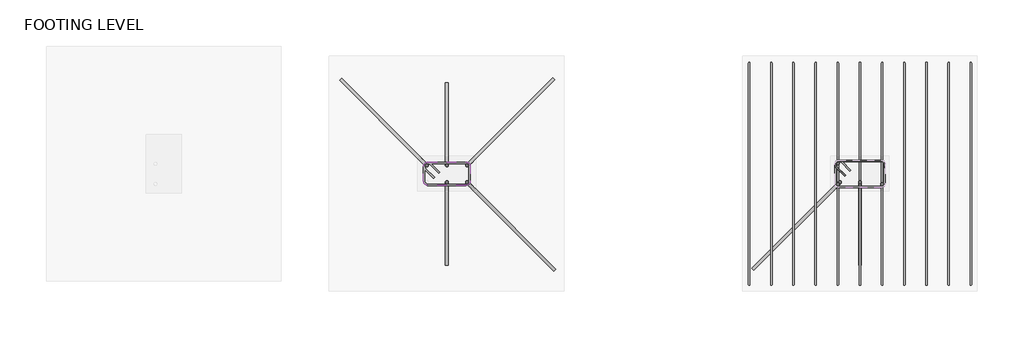
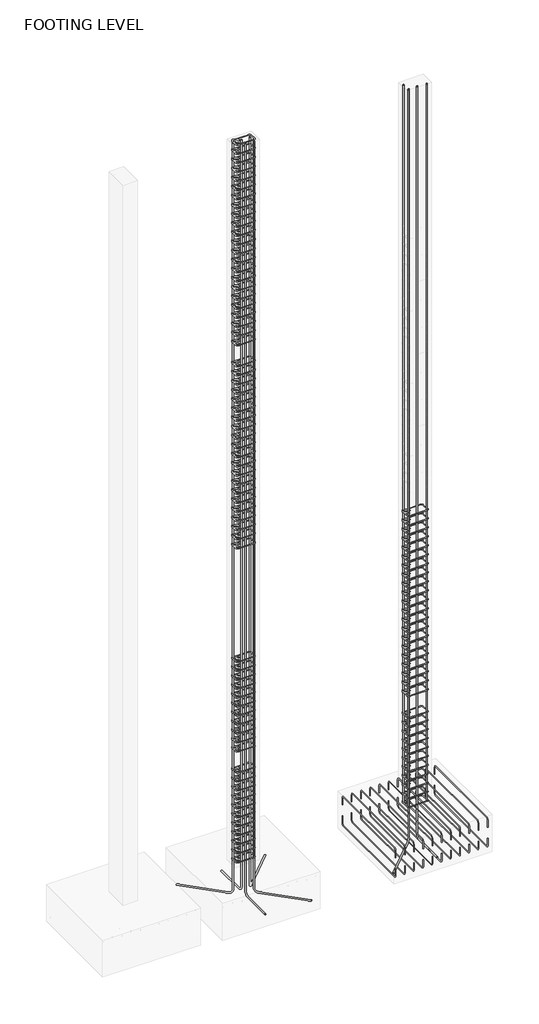
# One storey, part 4 of 10: 19 reinforcing bars.
"""IFC4 building model written with IfcOpenShell, lengths in millimetres."""

from ifc_helpers import new_model, si_unit, point, frame, origin, place, context, project, spatial, polyline, circle_curve, trimmed, segment, composite_curve, source, transform, mapped, element, save
from ifc_brep_helpers import swept_disk

model = new_model("IFC4")

# Units and contexts
model_context = context("Model", 3, world=origin())
ifc_project = project(units=[si_unit("LENGTHUNIT", "METRE", prefix="MILLI")], contexts=[model_context])

# Site, building, storey
site = spatial("IfcSite", under=ifc_project)
building = spatial("IfcBuilding", under=site)
storey = spatial("IfcBuildingStorey", under=building, Name="FOOTING LEVEL", Elevation=-1371.6)

# Reinforcing bars
placement = place(None, origin())
reinforcing_bar_shape = source(origin(), model_context, "Body", "SolidModel", [
    swept_disk(composite_curve([segment(polyline([(-10916.8793223, 5647.2626382, -1770.864029), (-10916.8793223, 5647.2626382, -1885.164029)]), True, "CONTINUOUS"), segment(trimmed(circle_curve(frame((-10916.8793223, 5613.9251382, -1885.164029), z_axis=(-1.0, 0.0, 0.0), x_axis=(0.0, 33.337499999999636, 0.0)), 33.3375), [point((-10916.8793223, 5647.2626382, -1885.164029))], [point((-10916.8793223, 5613.9251382, -1918.501529))], True, "CARTESIAN"), True, "CONTINUOUS"), segment(polyline([(-10916.8793223, 5613.9251382, -1918.501529), (-10916.8793223, 4242.3251382, -1918.501529)]), True, "CONTINUOUS"), segment(trimmed(circle_curve(frame((-10916.8793223, 4242.3251382, -1885.164029), z_axis=(-1.0, 0.0, 0.0), x_axis=(0.0, 0.0, -33.337499999999864)), 33.3375), [point((-10916.8793223, 4242.3251382, -1918.501529))], [point((-10916.8793223, 4208.9876382, -1885.164029))], True, "CARTESIAN"), True, "CONTINUOUS"), segment(polyline([(-10916.8793223, 4208.9876382, -1885.164029), (-10916.8793223, 4208.9876382, -1770.864029)]), True, "CONTINUOUS")], self_intersect=False), 4.7625),
])
element("IfcReinforcingBar", 1, at=placement, inside=storey, context=model_context, shape_type="MappedRepresentation", body=[
    mapped(reinforcing_bar_shape, transform((0.0, 0.0, 0.0), x_axis=(1.0, 0.0, 0.0), y_axis=(0.0, 1.0, 0.0), z_axis=(0.0, 0.0, 1.0))),
    mapped(reinforcing_bar_shape, transform((143.8275, 0.0, 0.0), x_axis=(1.0, 0.0, 0.0), y_axis=(0.0, 1.0, 0.0), z_axis=(0.0, 0.0, 1.0))),
    mapped(reinforcing_bar_shape, transform((287.655, 0.0, 0.0), x_axis=(1.0, 0.0, 0.0), y_axis=(0.0, 1.0, 0.0), z_axis=(0.0, 0.0, 1.0))),
    mapped(reinforcing_bar_shape, transform((431.4825, 0.0, 0.0), x_axis=(1.0, 0.0, 0.0), y_axis=(0.0, 1.0, 0.0), z_axis=(0.0, 0.0, 1.0))),
    mapped(reinforcing_bar_shape, transform((575.31, 0.0, 0.0), x_axis=(1.0, 0.0, 0.0), y_axis=(0.0, 1.0, 0.0), z_axis=(0.0, 0.0, 1.0))),
    mapped(reinforcing_bar_shape, transform((719.1375, 0.0, 0.0), x_axis=(1.0, 0.0, 0.0), y_axis=(0.0, 1.0, 0.0), z_axis=(0.0, 0.0, 1.0))),
    mapped(reinforcing_bar_shape, transform((862.965, 0.0, 0.0), x_axis=(1.0, 0.0, 0.0), y_axis=(0.0, 1.0, 0.0), z_axis=(0.0, 0.0, 1.0))),
    mapped(reinforcing_bar_shape, transform((1006.7925, 0.0, 0.0), x_axis=(1.0, 0.0, 0.0), y_axis=(0.0, 1.0, 0.0), z_axis=(0.0, 0.0, 1.0))),
    mapped(reinforcing_bar_shape, transform((1150.62, 0.0, 0.0), x_axis=(1.0, 0.0, 0.0), y_axis=(0.0, 1.0, 0.0), z_axis=(0.0, 0.0, 1.0))),
    mapped(reinforcing_bar_shape, transform((1294.4475, 0.0, 0.0), x_axis=(1.0, 0.0, 0.0), y_axis=(0.0, 1.0, 0.0), z_axis=(0.0, 0.0, 1.0))),
    mapped(reinforcing_bar_shape, transform((1438.275, 0.0, 0.0), x_axis=(1.0, 0.0, 0.0), y_axis=(0.0, 1.0, 0.0), z_axis=(0.0, 0.0, 1.0))),
])
reinforcing_bar_2_shape = source(origin(), model_context, "Body", "SolidModel", [
    swept_disk(composite_curve([segment(polyline([(-9478.6043223, 5647.2626382, -1586.5406765), (-9478.6043223, 5647.2626382, -1472.2406765)]), True, "CONTINUOUS"), segment(trimmed(circle_curve(frame((-9478.6043223, 5613.9251382, -1472.2406765), z_axis=(1.0, 0.0, 0.0), x_axis=(0.0, 33.337499999999636, 0.0)), 33.3375), [point((-9478.6043223, 5647.2626382, -1472.2406765))], [point((-9478.6043223, 5613.9251382, -1438.9031765))], True, "CARTESIAN"), True, "CONTINUOUS"), segment(polyline([(-9478.6043223, 5613.9251382, -1438.9031765), (-9478.6043223, 4242.3251382, -1438.9031765)]), True, "CONTINUOUS"), segment(trimmed(circle_curve(frame((-9478.6043223, 4242.3251382, -1472.2406765), z_axis=(1.0, 0.0, 0.0), x_axis=(0.0, 0.0, 33.33750000000009)), 33.3375), [point((-9478.6043223, 4242.3251382, -1438.9031765))], [point((-9478.6043223, 4208.9876382, -1472.2406765))], True, "CARTESIAN"), True, "CONTINUOUS"), segment(polyline([(-9478.6043223, 4208.9876382, -1472.2406765), (-9478.6043223, 4208.9876382, -1586.5406765)]), True, "CONTINUOUS")], self_intersect=False), 4.7625),
])
element("IfcReinforcingBar", 2, at=placement, inside=storey, context=model_context, shape_type="MappedRepresentation", body=[
    mapped(reinforcing_bar_2_shape, transform((0.0, 0.0, 0.0), x_axis=(1.0, 0.0, 0.0), y_axis=(0.0, 1.0, 0.0), z_axis=(0.0, 0.0, 1.0))),
    mapped(reinforcing_bar_2_shape, transform((-143.8275, 0.0, 0.0), x_axis=(1.0, 0.0, 0.0), y_axis=(0.0, 1.0, 0.0), z_axis=(0.0, 0.0, 1.0))),
    mapped(reinforcing_bar_2_shape, transform((-287.655, 0.0, 0.0), x_axis=(1.0, 0.0, 0.0), y_axis=(0.0, 1.0, 0.0), z_axis=(0.0, 0.0, 1.0))),
    mapped(reinforcing_bar_2_shape, transform((-431.4825, 0.0, 0.0), x_axis=(1.0, 0.0, 0.0), y_axis=(0.0, 1.0, 0.0), z_axis=(0.0, 0.0, 1.0))),
    mapped(reinforcing_bar_2_shape, transform((-575.31, 0.0, 0.0), x_axis=(1.0, 0.0, 0.0), y_axis=(0.0, 1.0, 0.0), z_axis=(0.0, 0.0, 1.0))),
    mapped(reinforcing_bar_2_shape, transform((-719.1375, 0.0, 0.0), x_axis=(1.0, 0.0, 0.0), y_axis=(0.0, 1.0, 0.0), z_axis=(0.0, 0.0, 1.0))),
    mapped(reinforcing_bar_2_shape, transform((-862.965, 0.0, 0.0), x_axis=(1.0, 0.0, 0.0), y_axis=(0.0, 1.0, 0.0), z_axis=(0.0, 0.0, 1.0))),
    mapped(reinforcing_bar_2_shape, transform((-1006.7925, 0.0, 0.0), x_axis=(1.0, 0.0, 0.0), y_axis=(0.0, 1.0, 0.0), z_axis=(0.0, 0.0, 1.0))),
    mapped(reinforcing_bar_2_shape, transform((-1150.62, 0.0, 0.0), x_axis=(1.0, 0.0, 0.0), y_axis=(0.0, 1.0, 0.0), z_axis=(0.0, 0.0, 1.0))),
    mapped(reinforcing_bar_2_shape, transform((-1294.4475, 0.0, 0.0), x_axis=(1.0, 0.0, 0.0), y_axis=(0.0, 1.0, 0.0), z_axis=(0.0, 0.0, 1.0))),
    mapped(reinforcing_bar_2_shape, transform((-1438.275, 0.0, 0.0), x_axis=(1.0, 0.0, 0.0), y_axis=(0.0, 1.0, 0.0), z_axis=(0.0, 0.0, 1.0))),
])
reinforcing_bar_3_shape = source(origin(), model_context, "Body", "SolidModel", [
    swept_disk(composite_curve([segment(polyline([(-10260.564645, 4948.4239213, -1337.3511872), (-10317.4288421, 5005.2881184, -1337.3511872)]), True, "CONTINUOUS"), segment(trimmed(circle_curve(frame((-10334.2668223, 4988.4501382, -1337.3511872), z_axis=(0.0, 0.0, 1.0), x_axis=(16.837980199999947, 16.837980199999947, 0.0)), 23.8125), [point((-10317.4288421, 5005.2881184, -1337.3511872))], [point((-10358.0793223, 4988.4501382, -1337.3511872))], True, "CARTESIAN"), True, "CONTINUOUS"), segment(polyline([(-10358.0793223, 4988.4501382, -1337.3511872), (-10358.0793223, 4867.8001382, -1337.3511872)]), True, "CONTINUOUS"), segment(trimmed(circle_curve(frame((-10334.2668223, 4867.8001382, -1337.3511872), z_axis=(0.0, 0.0, 1.0), x_axis=(-23.8125, 0.0, 0.0)), 23.8125), [point((-10358.0793223, 4867.8001382, -1337.3511872))], [point((-10334.2668223, 4843.9876382, -1337.3511872))], True, "CARTESIAN"), True, "CONTINUOUS"), segment(polyline([(-10334.2668223, 4843.9876382, -1337.3511872), (-10061.2168223, 4843.9876382, -1337.3511872)]), True, "CONTINUOUS"), segment(trimmed(circle_curve(frame((-10061.2168223, 4867.7620821, -1338.6969104), z_axis=(0.0, 0.056513312022656075, 0.9984018457335854), x_axis=(0.0, -23.774443899999824, 1.3457232000000658)), 23.8125), [point((-10061.2168223, 4843.9876382, -1337.3511872))], [point((-10037.4043223, 4867.7620821, -1338.6969104))], True, "CARTESIAN"), True, "CONTINUOUS"), segment(polyline([(-10037.4043223, 4867.7620821, -1338.6969104), (-10037.4043223, 4988.4881942, -1345.5304639)]), True, "CONTINUOUS"), segment(trimmed(circle_curve(frame((-10061.2168223, 4988.4881942, -1345.5304639), z_axis=(0.0, 0.056513312022656075, 0.9984018457335854), x_axis=(23.8125, 0.0, 0.0)), 23.8125), [point((-10037.4043223, 4988.4881942, -1345.5304639))], [point((-10061.2168223, 5012.2626382, -1346.8761872))], True, "CARTESIAN"), True, "CONTINUOUS"), segment(polyline([(-10061.2168223, 5012.2626382, -1346.8761872), (-10334.2668223, 5012.2626382, -1346.8761872)]), True, "CONTINUOUS"), segment(trimmed(circle_curve(frame((-10334.2668223, 4988.4501382, -1346.8761872), z_axis=(0.0, 0.0, 1.0), x_axis=(0.0, 23.8125, 0.0)), 23.8125), [point((-10334.2668223, 5012.2626382, -1346.8761872))], [point((-10351.1048026, 4971.6121579, -1346.8761872))], True, "CARTESIAN"), True, "CONTINUOUS"), segment(polyline([(-10351.1048026, 4971.6121579, -1346.8761872), (-10294.2406055, 4914.7479609, -1346.8761872)]), True, "CONTINUOUS")], self_intersect=False), 4.7625),
])
element("IfcReinforcingBar", 3, at=placement, inside=storey, context=model_context, shape_type="MappedRepresentation", body=[
    mapped(reinforcing_bar_3_shape, transform((0.0, 0.0, 0.0), x_axis=(1.0, 0.0, 0.0), y_axis=(0.0, 1.0, 0.0), z_axis=(0.0, 0.0, 1.0))),
    mapped(reinforcing_bar_3_shape, transform((0.0, 0.0, 147.1780014), x_axis=(1.0, 0.0, 0.0), y_axis=(0.0, 1.0, 0.0), z_axis=(0.0, 0.0, 1.0))),
    mapped(reinforcing_bar_3_shape, transform((0.0, 0.0, 294.3560028), x_axis=(1.0, 0.0, 0.0), y_axis=(0.0, 1.0, 0.0), z_axis=(0.0, 0.0, 1.0))),
    mapped(reinforcing_bar_3_shape, transform((0.0, 0.0, 441.5340042), x_axis=(1.0, 0.0, 0.0), y_axis=(0.0, 1.0, 0.0), z_axis=(0.0, 0.0, 1.0))),
    mapped(reinforcing_bar_3_shape, transform((0.0, 0.0, 588.7120056), x_axis=(1.0, 0.0, 0.0), y_axis=(0.0, 1.0, 0.0), z_axis=(0.0, 0.0, 1.0))),
    mapped(reinforcing_bar_3_shape, transform((0.0, 0.0, 735.890007), x_axis=(1.0, 0.0, 0.0), y_axis=(0.0, 1.0, 0.0), z_axis=(0.0, 0.0, 1.0))),
    mapped(reinforcing_bar_3_shape, transform((0.0, 0.0, 883.0680084), x_axis=(1.0, 0.0, 0.0), y_axis=(0.0, 1.0, 0.0), z_axis=(0.0, 0.0, 1.0))),
    mapped(reinforcing_bar_3_shape, transform((0.0, 0.0, 1030.2460098), x_axis=(1.0, 0.0, 0.0), y_axis=(0.0, 1.0, 0.0), z_axis=(0.0, 0.0, 1.0))),
    mapped(reinforcing_bar_3_shape, transform((0.0, 0.0, 1177.4240112), x_axis=(1.0, 0.0, 0.0), y_axis=(0.0, 1.0, 0.0), z_axis=(0.0, 0.0, 1.0))),
    mapped(reinforcing_bar_3_shape, transform((0.0, 0.0, 1324.6020126), x_axis=(1.0, 0.0, 0.0), y_axis=(0.0, 1.0, 0.0), z_axis=(0.0, 0.0, 1.0))),
    mapped(reinforcing_bar_3_shape, transform((0.0, 0.0, 1471.780014), x_axis=(1.0, 0.0, 0.0), y_axis=(0.0, 1.0, 0.0), z_axis=(0.0, 0.0, 1.0))),
])
element("IfcReinforcingBar", 4, at=placement, inside=storey, context=model_context, shape_type="SolidModel", body=[
    swept_disk(composite_curve([segment(polyline([(-10054.4816302, 4861.0649461, -1346.2), (-10054.4816302, 4861.0649461, 10490.2)]), True, "CONTINUOUS")], self_intersect=False), 9.525),
])
element("IfcReinforcingBar", 5, at=placement, inside=storey, context=model_context, shape_type="SolidModel", body=[
    swept_disk(composite_curve([segment(polyline([(-10341.0020144, 4995.1853303, -1346.2), (-10341.0020144, 4995.1853303, 10490.2)]), True, "CONTINUOUS")], self_intersect=False), 9.525),
])
element("IfcReinforcingBar", 6, at=placement, inside=storey, context=model_context, shape_type="SolidModel", body=[
    swept_disk(composite_curve([segment(polyline([(-10341.0020144, 4861.0649461, -1346.2), (-10341.0020144, 4861.0649461, 10490.2)]), True, "CONTINUOUS")], self_intersect=False), 9.525),
])
element("IfcReinforcingBar", 7, at=placement, inside=storey, context=model_context, shape_type="SolidModel", body=[
    swept_disk(composite_curve([segment(polyline([(-10892.4808347, 4309.5861258, -1910.4342608), (-10375.4483591, 4826.6186014, -1910.4342608)]), True, "CONTINUOUS"), segment(trimmed(circle_curve(frame((-10375.4483591, 4826.6186014, -1843.7592608), z_axis=(0.7071067811865229, -0.7071067811865721, 0.0), x_axis=(0.0, 0.0, -66.67499999999995)), 66.675), [point((-10375.4483591, 4826.6186014, -1910.4342608))], [point((-10328.3020144, 4873.7649461, -1843.7592608))], True, "CARTESIAN"), True, "CONTINUOUS"), segment(polyline([(-10328.3020144, 4873.7649461, -1843.7592608), (-10328.3020144, 4873.7649461, 10490.2)]), True, "CONTINUOUS")], self_intersect=False), 9.525),
])
element("IfcReinforcingBar", 8, at=placement, inside=storey, context=model_context, shape_type="SolidModel", body=[
    swept_disk(composite_curve([segment(polyline([(-10197.7418223, 4335.5350696, -1910.4342608), (-10197.7418223, 4807.0899461, -1910.4342608)]), True, "CONTINUOUS"), segment(trimmed(circle_curve(frame((-10197.7418223, 4807.0899461, -1843.7592608), z_axis=(1.0, 0.0, 0.0), x_axis=(0.0, 0.0, -66.67499999999995)), 66.675), [point((-10197.7418223, 4807.0899461, -1910.4342608))], [point((-10197.7418223, 4873.7649461, -1843.7592608))], True, "CARTESIAN"), True, "CONTINUOUS"), segment(polyline([(-10197.7418223, 4873.7649461, -1843.7592608), (-10197.7418223, 4873.7649461, 10490.2)]), True, "CONTINUOUS")], self_intersect=False), 9.525),
])
reinforcing_bar_4_shape = source(origin(), model_context, "Body", "SolidModel", [
    swept_disk(composite_curve([segment(polyline([(-12927.564645, 4935.7239213, -1328.7375), (-12984.4288421, 4992.5881184, -1328.7375)]), True, "CONTINUOUS"), segment(trimmed(circle_curve(frame((-13001.2668223, 4975.7501382, -1328.7375), z_axis=(0.0, 0.0, 1.0), x_axis=(16.837980199999947, 16.837980199999947, 0.0)), 23.8125), [point((-12984.4288421, 4992.5881184, -1328.7375))], [point((-13025.0793223, 4975.7501382, -1328.7375))], True, "CARTESIAN"), True, "CONTINUOUS"), segment(polyline([(-13025.0793223, 4975.7501382, -1328.7375), (-13025.0793223, 4880.5001382, -1328.7375)]), True, "CONTINUOUS"), segment(trimmed(circle_curve(frame((-13001.2668223, 4880.5001382, -1328.7375), z_axis=(0.0, 0.0, 1.0), x_axis=(-23.8125, 0.0, 0.0)), 23.8125), [point((-13025.0793223, 4880.5001382, -1328.7375))], [point((-13001.2668223, 4856.6876382, -1328.7375))], True, "CARTESIAN"), True, "CONTINUOUS"), segment(polyline([(-13001.2668223, 4856.6876382, -1328.7375), (-12753.6168223, 4856.6876382, -1328.7375)]), True, "CONTINUOUS"), segment(trimmed(circle_curve(frame((-12753.6168223, 4880.4473972, -1330.3214839), z_axis=(0.0, 0.06651901052377396, 0.9977851578566089), x_axis=(0.0, -23.759758999999576, 1.583983900000021)), 23.8125), [point((-12753.6168223, 4856.6876382, -1328.7375))], [point((-12729.8043223, 4880.4473972, -1330.3214839))], True, "CARTESIAN"), True, "CONTINUOUS"), segment(polyline([(-12729.8043223, 4880.4473972, -1330.3214839), (-12729.8043223, 4975.8028791, -1336.6785161)]), True, "CONTINUOUS"), segment(trimmed(circle_curve(frame((-12753.6168223, 4975.8028791, -1336.6785161), z_axis=(0.0, 0.06651901052377396, 0.9977851578566089), x_axis=(23.8125, 0.0, 0.0)), 23.8125), [point((-12729.8043223, 4975.8028791, -1336.6785161))], [point((-12753.6168223, 4999.5626382, -1338.2625))], True, "CARTESIAN"), True, "CONTINUOUS"), segment(polyline([(-12753.6168223, 4999.5626382, -1338.2625), (-13001.2668223, 4999.5626382, -1338.2625)]), True, "CONTINUOUS"), segment(trimmed(circle_curve(frame((-13001.2668223, 4975.7501382, -1338.2625), z_axis=(0.0, 0.0, 1.0), x_axis=(0.0, 23.8125, 0.0)), 23.8125), [point((-13001.2668223, 4999.5626382, -1338.2625))], [point((-13018.1048026, 4958.9121579, -1338.2625))], True, "CARTESIAN"), True, "CONTINUOUS"), segment(polyline([(-13018.1048026, 4958.9121579, -1338.2625), (-12961.2406055, 4902.0479609, -1338.2625)]), True, "CONTINUOUS")], self_intersect=False), 4.7625),
])
element("IfcReinforcingBar", 9, at=placement, inside=storey, context=model_context, shape_type="MappedRepresentation", body=[
    mapped(reinforcing_bar_4_shape, transform((0.0, 0.0, 0.0), x_axis=(1.0, 0.0, 0.0), y_axis=(0.0, 1.0, 0.0), z_axis=(0.0, 0.0, 1.0))),
    mapped(reinforcing_bar_4_shape, transform((0.0, 0.0, 148.11375), x_axis=(1.0, 0.0, 0.0), y_axis=(0.0, 1.0, 0.0), z_axis=(0.0, 0.0, 1.0))),
    mapped(reinforcing_bar_4_shape, transform((0.0, 0.0, 296.2275), x_axis=(1.0, 0.0, 0.0), y_axis=(0.0, 1.0, 0.0), z_axis=(0.0, 0.0, 1.0))),
    mapped(reinforcing_bar_4_shape, transform((0.0, 0.0, 444.34125), x_axis=(1.0, 0.0, 0.0), y_axis=(0.0, 1.0, 0.0), z_axis=(0.0, 0.0, 1.0))),
    mapped(reinforcing_bar_4_shape, transform((0.0, 0.0, 592.455), x_axis=(1.0, 0.0, 0.0), y_axis=(0.0, 1.0, 0.0), z_axis=(0.0, 0.0, 1.0))),
    mapped(reinforcing_bar_4_shape, transform((0.0, 0.0, 740.56875), x_axis=(1.0, 0.0, 0.0), y_axis=(0.0, 1.0, 0.0), z_axis=(0.0, 0.0, 1.0))),
    mapped(reinforcing_bar_4_shape, transform((0.0, 0.0, 888.6825), x_axis=(1.0, 0.0, 0.0), y_axis=(0.0, 1.0, 0.0), z_axis=(0.0, 0.0, 1.0))),
    mapped(reinforcing_bar_4_shape, transform((0.0, 0.0, 1036.79625), x_axis=(1.0, 0.0, 0.0), y_axis=(0.0, 1.0, 0.0), z_axis=(0.0, 0.0, 1.0))),
    mapped(reinforcing_bar_4_shape, transform((0.0, 0.0, 1184.91), x_axis=(1.0, 0.0, 0.0), y_axis=(0.0, 1.0, 0.0), z_axis=(0.0, 0.0, 1.0))),
    mapped(reinforcing_bar_4_shape, transform((0.0, 0.0, 1333.02375), x_axis=(1.0, 0.0, 0.0), y_axis=(0.0, 1.0, 0.0), z_axis=(0.0, 0.0, 1.0))),
    mapped(reinforcing_bar_4_shape, transform((0.0, 0.0, 1481.1375), x_axis=(1.0, 0.0, 0.0), y_axis=(0.0, 1.0, 0.0), z_axis=(0.0, 0.0, 1.0))),
])
element("IfcReinforcingBar", 10, at=placement, inside=storey, context=model_context, shape_type="SolidModel", body=[
    swept_disk(composite_curve([segment(polyline([(-12746.8816302, 4873.7649461, -1333.5), (-12746.8816302, 4873.7649461, 10477.5)]), True, "CONTINUOUS")], self_intersect=False), 9.525),
])
element("IfcReinforcingBar", 11, at=placement, inside=storey, context=model_context, shape_type="SolidModel", body=[
    swept_disk(composite_curve([segment(polyline([(-12185.2058743, 5544.1610861, -1910.4342608), (-12699.7352856, 5029.6316749, -1910.4342608)]), True, "CONTINUOUS"), segment(trimmed(circle_curve(frame((-12699.7352856, 5029.6316749, -1843.7592608), z_axis=(-0.7071067811865185, 0.7071067811865767, 0.0), x_axis=(0.0, 0.0, -66.67499999999995)), 66.675), [point((-12699.7352856, 5029.6316749, -1910.4342608))], [point((-12746.8816302, 4982.4853303, -1843.7592608))], True, "CARTESIAN"), True, "CONTINUOUS"), segment(polyline([(-12746.8816302, 4982.4853303, -1843.7592608), (-12746.8816302, 4982.4853303, 10477.5)]), True, "CONTINUOUS")], self_intersect=False), 9.525),
])
element("IfcReinforcingBar", 12, at=placement, inside=storey, context=model_context, shape_type="SolidModel", body=[
    swept_disk(composite_curve([segment(polyline([(-12177.1874965, 4304.0708123, -1910.4342608), (-12699.7352856, 4826.6186014, -1910.4342608)]), True, "CONTINUOUS"), segment(trimmed(circle_curve(frame((-12699.7352856, 4826.6186014, -1843.7592608), z_axis=(0.7071067811865269, 0.7071067811865681, 0.0), x_axis=(0.0, 0.0, -66.67499999999995)), 66.675), [point((-12699.7352856, 4826.6186014, -1910.4342608))], [point((-12746.8816302, 4873.7649461, -1843.7592608))], True, "CARTESIAN"), True, "CONTINUOUS"), segment(polyline([(-12746.8816302, 4873.7649461, -1843.7592608), (-12746.8816302, 4873.7649461, 10477.5)]), True, "CONTINUOUS")], self_intersect=False), 9.525),
])
element("IfcReinforcingBar", 13, at=placement, inside=storey, context=model_context, shape_type="SolidModel", body=[
    swept_disk(composite_curve([segment(polyline([(-13566.7211349, 5541.2044507, -1910.4342608), (-13055.1483591, 5029.6316749, -1910.4342608)]), True, "CONTINUOUS"), segment(trimmed(circle_curve(frame((-13055.1483591, 5029.6316749, -1843.7592608), z_axis=(-0.7071067811865223, -0.7071067811865729, 0.0), x_axis=(0.0, 0.0, -66.67499999999995)), 66.675), [point((-13055.1483591, 5029.6316749, -1910.4342608))], [point((-13008.0020144, 4982.4853303, -1843.7592608))], True, "CARTESIAN"), True, "CONTINUOUS"), segment(polyline([(-13008.0020144, 4982.4853303, -1843.7592608), (-13008.0020144, 4982.4853303, 10477.5)]), True, "CONTINUOUS")], self_intersect=False), 9.525),
])
element("IfcReinforcingBar", 14, at=placement, inside=storey, context=model_context, shape_type="SolidModel", body=[
    swept_disk(composite_curve([segment(polyline([(-12877.4418223, 5520.7152067, -1910.4342608), (-12877.4418223, 5049.1603303, -1910.4342608)]), True, "CONTINUOUS"), segment(trimmed(circle_curve(frame((-12877.4418223, 5049.1603303, -1843.7592608), z_axis=(-1.0, 0.0, 0.0), x_axis=(0.0, 0.0, -66.67499999999995)), 66.675), [point((-12877.4418223, 5049.1603303, -1910.4342608))], [point((-12877.4418223, 4982.4853303, -1843.7592608))], True, "CARTESIAN"), True, "CONTINUOUS"), segment(polyline([(-12877.4418223, 4982.4853303, -1843.7592608), (-12877.4418223, 4982.4853303, 10477.5)]), True, "CONTINUOUS")], self_intersect=False), 9.525),
])
element("IfcReinforcingBar", 15, at=placement, inside=storey, context=model_context, shape_type="SolidModel", body=[
    swept_disk(composite_curve([segment(polyline([(-12877.4418223, 4335.5350696, -1910.4342608), (-12877.4418223, 4807.0899461, -1910.4342608)]), True, "CONTINUOUS"), segment(trimmed(circle_curve(frame((-12877.4418223, 4807.0899461, -1843.7592608), z_axis=(1.0, 0.0, 0.0), x_axis=(0.0, 0.0, -66.67499999999995)), 66.675), [point((-12877.4418223, 4807.0899461, -1910.4342608))], [point((-12877.4418223, 4873.7649461, -1843.7592608))], True, "CARTESIAN"), True, "CONTINUOUS"), segment(polyline([(-12877.4418223, 4873.7649461, -1843.7592608), (-12877.4418223, 4873.7649461, 10477.5)]), True, "CONTINUOUS")], self_intersect=False), 9.525),
])
reinforcing_bar_5_shape = source(origin(), model_context, "Body", "SolidModel", [
    swept_disk(composite_curve([segment(polyline([(-10260.564645, 4948.4239213, 491.4488128), (-10317.4288421, 5005.2881184, 491.4488128)]), True, "CONTINUOUS"), segment(trimmed(circle_curve(frame((-10334.2668223, 4988.4501382, 491.4488128), z_axis=(0.0, 0.0, 1.0), x_axis=(16.837980199999947, 16.837980199999947, 0.0)), 23.8125), [point((-10317.4288421, 5005.2881184, 491.4488128))], [point((-10358.0793223, 4988.4501382, 491.4488128))], True, "CARTESIAN"), True, "CONTINUOUS"), segment(polyline([(-10358.0793223, 4988.4501382, 491.4488128), (-10358.0793223, 4867.8001382, 491.4488128)]), True, "CONTINUOUS"), segment(trimmed(circle_curve(frame((-10334.2668223, 4867.8001382, 491.4488128), z_axis=(0.0, 0.0, 1.0), x_axis=(-23.8125, 0.0, 0.0)), 23.8125), [point((-10358.0793223, 4867.8001382, 491.4488128))], [point((-10334.2668223, 4843.9876382, 491.4488128))], True, "CARTESIAN"), True, "CONTINUOUS"), segment(polyline([(-10334.2668223, 4843.9876382, 491.4488128), (-10061.2168223, 4843.9876382, 491.4488128)]), True, "CONTINUOUS"), segment(trimmed(circle_curve(frame((-10061.2168223, 4867.7620821, 490.1030896), z_axis=(0.0, 0.056513312022656075, 0.9984018457335854), x_axis=(0.0, -23.774443899999824, 1.345723200000009)), 23.8125), [point((-10061.2168223, 4843.9876382, 491.4488128))], [point((-10037.4043223, 4867.7620821, 490.1030896))], True, "CARTESIAN"), True, "CONTINUOUS"), segment(polyline([(-10037.4043223, 4867.7620821, 490.1030896), (-10037.4043223, 4988.4881942, 483.2695361)]), True, "CONTINUOUS"), segment(trimmed(circle_curve(frame((-10061.2168223, 4988.4881942, 483.2695361), z_axis=(0.0, 0.056513312022656075, 0.9984018457335854), x_axis=(23.8125, 0.0, 0.0)), 23.8125), [point((-10037.4043223, 4988.4881942, 483.2695361))], [point((-10061.2168223, 5012.2626382, 481.9238128))], True, "CARTESIAN"), True, "CONTINUOUS"), segment(polyline([(-10061.2168223, 5012.2626382, 481.9238128), (-10334.2668223, 5012.2626382, 481.9238128)]), True, "CONTINUOUS"), segment(trimmed(circle_curve(frame((-10334.2668223, 4988.4501382, 481.9238128), z_axis=(0.0, 0.0, 1.0), x_axis=(0.0, 23.8125, 0.0)), 23.8125), [point((-10334.2668223, 5012.2626382, 481.9238128))], [point((-10351.1048026, 4971.6121579, 481.9238128))], True, "CARTESIAN"), True, "CONTINUOUS"), segment(polyline([(-10351.1048026, 4971.6121579, 481.9238128), (-10294.2406055, 4914.7479609, 481.9238128)]), True, "CONTINUOUS")], self_intersect=False), 4.7625),
])
element("IfcReinforcingBar", 16, at=placement, inside=storey, context=model_context, shape_type="MappedRepresentation", body=[
    mapped(reinforcing_bar_5_shape, transform((0.0, 0.0, 0.0), x_axis=(1.0, 0.0, 0.0), y_axis=(0.0, 1.0, 0.0), z_axis=(0.0, 0.0, 1.0))),
    mapped(reinforcing_bar_5_shape, transform((0.0, 0.0, 148.5671059), x_axis=(1.0, 0.0, 0.0), y_axis=(0.0, 1.0, 0.0), z_axis=(0.0, 0.0, 1.0))),
    mapped(reinforcing_bar_5_shape, transform((0.0, 0.0, 297.1342118), x_axis=(1.0, 0.0, 0.0), y_axis=(0.0, 1.0, 0.0), z_axis=(0.0, 0.0, 1.0))),
    mapped(reinforcing_bar_5_shape, transform((0.0, 0.0, 445.7013177), x_axis=(1.0, 0.0, 0.0), y_axis=(0.0, 1.0, 0.0), z_axis=(0.0, 0.0, 1.0))),
    mapped(reinforcing_bar_5_shape, transform((0.0, 0.0, 594.2684236), x_axis=(1.0, 0.0, 0.0), y_axis=(0.0, 1.0, 0.0), z_axis=(0.0, 0.0, 1.0))),
    mapped(reinforcing_bar_5_shape, transform((0.0, 0.0, 742.8355295), x_axis=(1.0, 0.0, 0.0), y_axis=(0.0, 1.0, 0.0), z_axis=(0.0, 0.0, 1.0))),
    mapped(reinforcing_bar_5_shape, transform((0.0, 0.0, 891.4026354), x_axis=(1.0, 0.0, 0.0), y_axis=(0.0, 1.0, 0.0), z_axis=(0.0, 0.0, 1.0))),
    mapped(reinforcing_bar_5_shape, transform((0.0, 0.0, 1039.9697413), x_axis=(1.0, 0.0, 0.0), y_axis=(0.0, 1.0, 0.0), z_axis=(0.0, 0.0, 1.0))),
    mapped(reinforcing_bar_5_shape, transform((0.0, 0.0, 1188.5368472), x_axis=(1.0, 0.0, 0.0), y_axis=(0.0, 1.0, 0.0), z_axis=(0.0, 0.0, 1.0))),
    mapped(reinforcing_bar_5_shape, transform((0.0, 0.0, 1337.1039531), x_axis=(1.0, 0.0, 0.0), y_axis=(0.0, 1.0, 0.0), z_axis=(0.0, 0.0, 1.0))),
    mapped(reinforcing_bar_5_shape, transform((0.0, 0.0, 1485.671059), x_axis=(1.0, 0.0, 0.0), y_axis=(0.0, 1.0, 0.0), z_axis=(0.0, 0.0, 1.0))),
    mapped(reinforcing_bar_5_shape, transform((0.0, 0.0, 1634.2381649), x_axis=(1.0, 0.0, 0.0), y_axis=(0.0, 1.0, 0.0), z_axis=(0.0, 0.0, 1.0))),
    mapped(reinforcing_bar_5_shape, transform((0.0, 0.0, 1782.8052708), x_axis=(1.0, 0.0, 0.0), y_axis=(0.0, 1.0, 0.0), z_axis=(0.0, 0.0, 1.0))),
    mapped(reinforcing_bar_5_shape, transform((0.0, 0.0, 1931.3723767), x_axis=(1.0, 0.0, 0.0), y_axis=(0.0, 1.0, 0.0), z_axis=(0.0, 0.0, 1.0))),
    mapped(reinforcing_bar_5_shape, transform((0.0, 0.0, 2079.9394826), x_axis=(1.0, 0.0, 0.0), y_axis=(0.0, 1.0, 0.0), z_axis=(0.0, 0.0, 1.0))),
    mapped(reinforcing_bar_5_shape, transform((0.0, 0.0, 2228.5065885), x_axis=(1.0, 0.0, 0.0), y_axis=(0.0, 1.0, 0.0), z_axis=(0.0, 0.0, 1.0))),
    mapped(reinforcing_bar_5_shape, transform((0.0, 0.0, 2377.0736944), x_axis=(1.0, 0.0, 0.0), y_axis=(0.0, 1.0, 0.0), z_axis=(0.0, 0.0, 1.0))),
    mapped(reinforcing_bar_5_shape, transform((0.0, 0.0, 2525.6408003), x_axis=(1.0, 0.0, 0.0), y_axis=(0.0, 1.0, 0.0), z_axis=(0.0, 0.0, 1.0))),
    mapped(reinforcing_bar_5_shape, transform((0.0, 0.0, 2674.2079062), x_axis=(1.0, 0.0, 0.0), y_axis=(0.0, 1.0, 0.0), z_axis=(0.0, 0.0, 1.0))),
    mapped(reinforcing_bar_5_shape, transform((0.0, 0.0, 2822.775012), x_axis=(1.0, 0.0, 0.0), y_axis=(0.0, 1.0, 0.0), z_axis=(0.0, 0.0, 1.0))),
    mapped(reinforcing_bar_5_shape, transform((0.0, 0.0, 2971.3421179), x_axis=(1.0, 0.0, 0.0), y_axis=(0.0, 1.0, 0.0), z_axis=(0.0, 0.0, 1.0))),
])
reinforcing_bar_6_shape = source(origin(), model_context, "Body", "SolidModel", [
    swept_disk(composite_curve([segment(polyline([(-12927.564645, 4935.7239213, 500.0625), (-12984.4288421, 4992.5881184, 500.0625)]), True, "CONTINUOUS"), segment(trimmed(circle_curve(frame((-13001.2668223, 4975.7501382, 500.0625), z_axis=(0.0, 0.0, 1.0), x_axis=(16.837980199999947, 16.837980199999947, 0.0)), 23.8125), [point((-12984.4288421, 4992.5881184, 500.0625))], [point((-13025.0793223, 4975.7501382, 500.0625))], True, "CARTESIAN"), True, "CONTINUOUS"), segment(polyline([(-13025.0793223, 4975.7501382, 500.0625), (-13025.0793223, 4880.5001382, 500.0625)]), True, "CONTINUOUS"), segment(trimmed(circle_curve(frame((-13001.2668223, 4880.5001382, 500.0625), z_axis=(0.0, 0.0, 1.0), x_axis=(-23.8125, 0.0, 0.0)), 23.8125), [point((-13025.0793223, 4880.5001382, 500.0625))], [point((-13001.2668223, 4856.6876382, 500.0625))], True, "CARTESIAN"), True, "CONTINUOUS"), segment(polyline([(-13001.2668223, 4856.6876382, 500.0625), (-12753.6168223, 4856.6876382, 500.0625)]), True, "CONTINUOUS"), segment(trimmed(circle_curve(frame((-12753.6168223, 4880.4473972, 498.4785161), z_axis=(0.0, 0.06651901052377396, 0.9977851578566089), x_axis=(0.0, -23.759758999999576, 1.583983900000021)), 23.8125), [point((-12753.6168223, 4856.6876382, 500.0625))], [point((-12729.8043223, 4880.4473972, 498.4785161))], True, "CARTESIAN"), True, "CONTINUOUS"), segment(polyline([(-12729.8043223, 4880.4473972, 498.4785161), (-12729.8043223, 4975.8028791, 492.1214839)]), True, "CONTINUOUS"), segment(trimmed(circle_curve(frame((-12753.6168223, 4975.8028791, 492.1214839), z_axis=(0.0, 0.06651901052377396, 0.9977851578566089), x_axis=(23.8125, 0.0, 0.0)), 23.8125), [point((-12729.8043223, 4975.8028791, 492.1214839))], [point((-12753.6168223, 4999.5626382, 490.5375))], True, "CARTESIAN"), True, "CONTINUOUS"), segment(polyline([(-12753.6168223, 4999.5626382, 490.5375), (-13001.2668223, 4999.5626382, 490.5375)]), True, "CONTINUOUS"), segment(trimmed(circle_curve(frame((-13001.2668223, 4975.7501382, 490.5375), z_axis=(0.0, 0.0, 1.0), x_axis=(0.0, 23.8125, 0.0)), 23.8125), [point((-13001.2668223, 4999.5626382, 490.5375))], [point((-13018.1048026, 4958.9121579, 490.5375))], True, "CARTESIAN"), True, "CONTINUOUS"), segment(polyline([(-13018.1048026, 4958.9121579, 490.5375), (-12961.2406055, 4902.0479609, 490.5375)]), True, "CONTINUOUS")], self_intersect=False), 4.7625),
])
element("IfcReinforcingBar", 17, at=placement, inside=storey, context=model_context, shape_type="MappedRepresentation", body=[
    mapped(reinforcing_bar_6_shape, transform((0.0, 0.0, 0.0), x_axis=(1.0, 0.0, 0.0), y_axis=(0.0, 1.0, 0.0), z_axis=(0.0, 0.0, 1.0))),
    mapped(reinforcing_bar_6_shape, transform((0.0, 0.0, 148.11375), x_axis=(1.0, 0.0, 0.0), y_axis=(0.0, 1.0, 0.0), z_axis=(0.0, 0.0, 1.0))),
    mapped(reinforcing_bar_6_shape, transform((0.0, 0.0, 296.2275), x_axis=(1.0, 0.0, 0.0), y_axis=(0.0, 1.0, 0.0), z_axis=(0.0, 0.0, 1.0))),
    mapped(reinforcing_bar_6_shape, transform((0.0, 0.0, 444.34125), x_axis=(1.0, 0.0, 0.0), y_axis=(0.0, 1.0, 0.0), z_axis=(0.0, 0.0, 1.0))),
    mapped(reinforcing_bar_6_shape, transform((0.0, 0.0, 592.455), x_axis=(1.0, 0.0, 0.0), y_axis=(0.0, 1.0, 0.0), z_axis=(0.0, 0.0, 1.0))),
    mapped(reinforcing_bar_6_shape, transform((0.0, 0.0, 740.56875), x_axis=(1.0, 0.0, 0.0), y_axis=(0.0, 1.0, 0.0), z_axis=(0.0, 0.0, 1.0))),
    mapped(reinforcing_bar_6_shape, transform((0.0, 0.0, 888.6825), x_axis=(1.0, 0.0, 0.0), y_axis=(0.0, 1.0, 0.0), z_axis=(0.0, 0.0, 1.0))),
    mapped(reinforcing_bar_6_shape, transform((0.0, 0.0, 1036.79625), x_axis=(1.0, 0.0, 0.0), y_axis=(0.0, 1.0, 0.0), z_axis=(0.0, 0.0, 1.0))),
    mapped(reinforcing_bar_6_shape, transform((0.0, 0.0, 1184.91), x_axis=(1.0, 0.0, 0.0), y_axis=(0.0, 1.0, 0.0), z_axis=(0.0, 0.0, 1.0))),
    mapped(reinforcing_bar_6_shape, transform((0.0, 0.0, 1333.02375), x_axis=(1.0, 0.0, 0.0), y_axis=(0.0, 1.0, 0.0), z_axis=(0.0, 0.0, 1.0))),
    mapped(reinforcing_bar_6_shape, transform((0.0, 0.0, 1481.1375), x_axis=(1.0, 0.0, 0.0), y_axis=(0.0, 1.0, 0.0), z_axis=(0.0, 0.0, 1.0))),
])
reinforcing_bar_7_shape = source(origin(), model_context, "Body", "SolidModel", [
    swept_disk(composite_curve([segment(polyline([(-12927.564645, 4935.7239213, 3852.8625), (-12984.4288421, 4992.5881184, 3852.8625)]), True, "CONTINUOUS"), segment(trimmed(circle_curve(frame((-13001.2668223, 4975.7501382, 3852.8625), z_axis=(0.0, 0.0, 1.0), x_axis=(16.837980199999947, 16.837980199999947, 0.0)), 23.8125), [point((-12984.4288421, 4992.5881184, 3852.8625))], [point((-13025.0793223, 4975.7501382, 3852.8625))], True, "CARTESIAN"), True, "CONTINUOUS"), segment(polyline([(-13025.0793223, 4975.7501382, 3852.8625), (-13025.0793223, 4880.5001382, 3852.8625)]), True, "CONTINUOUS"), segment(trimmed(circle_curve(frame((-13001.2668223, 4880.5001382, 3852.8625), z_axis=(0.0, 0.0, 1.0), x_axis=(-23.8125, 0.0, 0.0)), 23.8125), [point((-13025.0793223, 4880.5001382, 3852.8625))], [point((-13001.2668223, 4856.6876382, 3852.8625))], True, "CARTESIAN"), True, "CONTINUOUS"), segment(polyline([(-13001.2668223, 4856.6876382, 3852.8625), (-12753.6168223, 4856.6876382, 3852.8625)]), True, "CONTINUOUS"), segment(trimmed(circle_curve(frame((-12753.6168223, 4880.4473972, 3851.2785161), z_axis=(0.0, 0.06651901052377396, 0.9977851578566089), x_axis=(0.0, -23.759758999999576, 1.583983900000021)), 23.8125), [point((-12753.6168223, 4856.6876382, 3852.8625))], [point((-12729.8043223, 4880.4473972, 3851.2785161))], True, "CARTESIAN"), True, "CONTINUOUS"), segment(polyline([(-12729.8043223, 4880.4473972, 3851.2785161), (-12729.8043223, 4975.8028791, 3844.9214839)]), True, "CONTINUOUS"), segment(trimmed(circle_curve(frame((-12753.6168223, 4975.8028791, 3844.9214839), z_axis=(0.0, 0.06651901052377396, 0.9977851578566089), x_axis=(23.8125, 0.0, 0.0)), 23.8125), [point((-12729.8043223, 4975.8028791, 3844.9214839))], [point((-12753.6168223, 4999.5626382, 3843.3375))], True, "CARTESIAN"), True, "CONTINUOUS"), segment(polyline([(-12753.6168223, 4999.5626382, 3843.3375), (-13001.2668223, 4999.5626382, 3843.3375)]), True, "CONTINUOUS"), segment(trimmed(circle_curve(frame((-13001.2668223, 4975.7501382, 3843.3375), z_axis=(0.0, 0.0, 1.0), x_axis=(0.0, 23.8125, 0.0)), 23.8125), [point((-13001.2668223, 4999.5626382, 3843.3375))], [point((-13018.1048026, 4958.9121579, 3843.3375))], True, "CARTESIAN"), True, "CONTINUOUS"), segment(polyline([(-13018.1048026, 4958.9121579, 3843.3375), (-12961.2406055, 4902.0479609, 3843.3375)]), True, "CONTINUOUS")], self_intersect=False), 4.7625),
])
element("IfcReinforcingBar", 18, at=placement, inside=storey, context=model_context, shape_type="MappedRepresentation", body=[
    mapped(reinforcing_bar_7_shape, transform((0.0, 0.0, 0.0), x_axis=(1.0, 0.0, 0.0), y_axis=(0.0, 1.0, 0.0), z_axis=(0.0, 0.0, 1.0))),
    mapped(reinforcing_bar_7_shape, transform((0.0, 0.0, 150.256875), x_axis=(1.0, 0.0, 0.0), y_axis=(0.0, 1.0, 0.0), z_axis=(0.0, 0.0, 1.0))),
    mapped(reinforcing_bar_7_shape, transform((0.0, 0.0, 300.51375), x_axis=(1.0, 0.0, 0.0), y_axis=(0.0, 1.0, 0.0), z_axis=(0.0, 0.0, 1.0))),
    mapped(reinforcing_bar_7_shape, transform((0.0, 0.0, 450.770625), x_axis=(1.0, 0.0, 0.0), y_axis=(0.0, 1.0, 0.0), z_axis=(0.0, 0.0, 1.0))),
    mapped(reinforcing_bar_7_shape, transform((0.0, 0.0, 601.0275), x_axis=(1.0, 0.0, 0.0), y_axis=(0.0, 1.0, 0.0), z_axis=(0.0, 0.0, 1.0))),
    mapped(reinforcing_bar_7_shape, transform((0.0, 0.0, 751.284375), x_axis=(1.0, 0.0, 0.0), y_axis=(0.0, 1.0, 0.0), z_axis=(0.0, 0.0, 1.0))),
    mapped(reinforcing_bar_7_shape, transform((0.0, 0.0, 901.54125), x_axis=(1.0, 0.0, 0.0), y_axis=(0.0, 1.0, 0.0), z_axis=(0.0, 0.0, 1.0))),
    mapped(reinforcing_bar_7_shape, transform((0.0, 0.0, 1051.798125), x_axis=(1.0, 0.0, 0.0), y_axis=(0.0, 1.0, 0.0), z_axis=(0.0, 0.0, 1.0))),
    mapped(reinforcing_bar_7_shape, transform((0.0, 0.0, 1202.055), x_axis=(1.0, 0.0, 0.0), y_axis=(0.0, 1.0, 0.0), z_axis=(0.0, 0.0, 1.0))),
    mapped(reinforcing_bar_7_shape, transform((0.0, 0.0, 1352.311875), x_axis=(1.0, 0.0, 0.0), y_axis=(0.0, 1.0, 0.0), z_axis=(0.0, 0.0, 1.0))),
    mapped(reinforcing_bar_7_shape, transform((0.0, 0.0, 1502.56875), x_axis=(1.0, 0.0, 0.0), y_axis=(0.0, 1.0, 0.0), z_axis=(0.0, 0.0, 1.0))),
    mapped(reinforcing_bar_7_shape, transform((0.0, 0.0, 1652.825625), x_axis=(1.0, 0.0, 0.0), y_axis=(0.0, 1.0, 0.0), z_axis=(0.0, 0.0, 1.0))),
    mapped(reinforcing_bar_7_shape, transform((0.0, 0.0, 1803.0825), x_axis=(1.0, 0.0, 0.0), y_axis=(0.0, 1.0, 0.0), z_axis=(0.0, 0.0, 1.0))),
    mapped(reinforcing_bar_7_shape, transform((0.0, 0.0, 1953.339375), x_axis=(1.0, 0.0, 0.0), y_axis=(0.0, 1.0, 0.0), z_axis=(0.0, 0.0, 1.0))),
    mapped(reinforcing_bar_7_shape, transform((0.0, 0.0, 2103.59625), x_axis=(1.0, 0.0, 0.0), y_axis=(0.0, 1.0, 0.0), z_axis=(0.0, 0.0, 1.0))),
    mapped(reinforcing_bar_7_shape, transform((0.0, 0.0, 2253.853125), x_axis=(1.0, 0.0, 0.0), y_axis=(0.0, 1.0, 0.0), z_axis=(0.0, 0.0, 1.0))),
    mapped(reinforcing_bar_7_shape, transform((0.0, 0.0, 2404.11), x_axis=(1.0, 0.0, 0.0), y_axis=(0.0, 1.0, 0.0), z_axis=(0.0, 0.0, 1.0))),
    mapped(reinforcing_bar_7_shape, transform((0.0, 0.0, 2554.366875), x_axis=(1.0, 0.0, 0.0), y_axis=(0.0, 1.0, 0.0), z_axis=(0.0, 0.0, 1.0))),
    mapped(reinforcing_bar_7_shape, transform((0.0, 0.0, 2704.62375), x_axis=(1.0, 0.0, 0.0), y_axis=(0.0, 1.0, 0.0), z_axis=(0.0, 0.0, 1.0))),
    mapped(reinforcing_bar_7_shape, transform((0.0, 0.0, 2854.880625), x_axis=(1.0, 0.0, 0.0), y_axis=(0.0, 1.0, 0.0), z_axis=(0.0, 0.0, 1.0))),
    mapped(reinforcing_bar_7_shape, transform((0.0, 0.0, 3005.1375), x_axis=(1.0, 0.0, 0.0), y_axis=(0.0, 1.0, 0.0), z_axis=(0.0, 0.0, 1.0))),
])
reinforcing_bar_8_shape = source(origin(), model_context, "Body", "SolidModel", [
    swept_disk(composite_curve([segment(polyline([(-12927.564645, 4935.7239213, 7205.6625), (-12984.4288421, 4992.5881184, 7205.6625)]), True, "CONTINUOUS"), segment(trimmed(circle_curve(frame((-13001.2668223, 4975.7501382, 7205.6625), z_axis=(0.0, 0.0, 1.0), x_axis=(16.837980199999947, 16.837980199999947, 0.0)), 23.8125), [point((-12984.4288421, 4992.5881184, 7205.6625))], [point((-13025.0793223, 4975.7501382, 7205.6625))], True, "CARTESIAN"), True, "CONTINUOUS"), segment(polyline([(-13025.0793223, 4975.7501382, 7205.6625), (-13025.0793223, 4880.5001382, 7205.6625)]), True, "CONTINUOUS"), segment(trimmed(circle_curve(frame((-13001.2668223, 4880.5001382, 7205.6625), z_axis=(0.0, 0.0, 1.0), x_axis=(-23.8125, 0.0, 0.0)), 23.8125), [point((-13025.0793223, 4880.5001382, 7205.6625))], [point((-13001.2668223, 4856.6876382, 7205.6625))], True, "CARTESIAN"), True, "CONTINUOUS"), segment(polyline([(-13001.2668223, 4856.6876382, 7205.6625), (-12753.6168223, 4856.6876382, 7205.6625)]), True, "CONTINUOUS"), segment(trimmed(circle_curve(frame((-12753.6168223, 4880.4473972, 7204.0785161), z_axis=(0.0, 0.06651901052377396, 0.9977851578566089), x_axis=(0.0, -23.759758999999576, 1.583983900000021)), 23.8125), [point((-12753.6168223, 4856.6876382, 7205.6625))], [point((-12729.8043223, 4880.4473972, 7204.0785161))], True, "CARTESIAN"), True, "CONTINUOUS"), segment(polyline([(-12729.8043223, 4880.4473972, 7204.0785161), (-12729.8043223, 4975.8028791, 7197.7214839)]), True, "CONTINUOUS"), segment(trimmed(circle_curve(frame((-12753.6168223, 4975.8028791, 7197.7214839), z_axis=(0.0, 0.06651901052377396, 0.9977851578566089), x_axis=(23.8125, 0.0, 0.0)), 23.8125), [point((-12729.8043223, 4975.8028791, 7197.7214839))], [point((-12753.6168223, 4999.5626382, 7196.1375))], True, "CARTESIAN"), True, "CONTINUOUS"), segment(polyline([(-12753.6168223, 4999.5626382, 7196.1375), (-13001.2668223, 4999.5626382, 7196.1375)]), True, "CONTINUOUS"), segment(trimmed(circle_curve(frame((-13001.2668223, 4975.7501382, 7196.1375), z_axis=(0.0, 0.0, 1.0), x_axis=(0.0, 23.8125, 0.0)), 23.8125), [point((-13001.2668223, 4999.5626382, 7196.1375))], [point((-13018.1048026, 4958.9121579, 7196.1375))], True, "CARTESIAN"), True, "CONTINUOUS"), segment(polyline([(-13018.1048026, 4958.9121579, 7196.1375), (-12961.2406055, 4902.0479609, 7196.1375)]), True, "CONTINUOUS")], self_intersect=False), 4.7625),
])
element("IfcReinforcingBar", 19, at=placement, inside=storey, context=model_context, shape_type="MappedRepresentation", body=[
    mapped(reinforcing_bar_8_shape, transform((0.0, 0.0, 0.0), x_axis=(1.0, 0.0, 0.0), y_axis=(0.0, 1.0, 0.0), z_axis=(0.0, 0.0, 1.0))),
    mapped(reinforcing_bar_8_shape, transform((0.0, 0.0, 150.4517045), x_axis=(1.0, 0.0, 0.0), y_axis=(0.0, 1.0, 0.0), z_axis=(0.0, 0.0, 1.0))),
    mapped(reinforcing_bar_8_shape, transform((0.0, 0.0, 300.9034091), x_axis=(1.0, 0.0, 0.0), y_axis=(0.0, 1.0, 0.0), z_axis=(0.0, 0.0, 1.0))),
    mapped(reinforcing_bar_8_shape, transform((0.0, 0.0, 451.3551136), x_axis=(1.0, 0.0, 0.0), y_axis=(0.0, 1.0, 0.0), z_axis=(0.0, 0.0, 1.0))),
    mapped(reinforcing_bar_8_shape, transform((0.0, 0.0, 601.8068182), x_axis=(1.0, 0.0, 0.0), y_axis=(0.0, 1.0, 0.0), z_axis=(0.0, 0.0, 1.0))),
    mapped(reinforcing_bar_8_shape, transform((0.0, 0.0, 752.2585227), x_axis=(1.0, 0.0, 0.0), y_axis=(0.0, 1.0, 0.0), z_axis=(0.0, 0.0, 1.0))),
    mapped(reinforcing_bar_8_shape, transform((0.0, 0.0, 902.7102273), x_axis=(1.0, 0.0, 0.0), y_axis=(0.0, 1.0, 0.0), z_axis=(0.0, 0.0, 1.0))),
    mapped(reinforcing_bar_8_shape, transform((0.0, 0.0, 1053.1619318), x_axis=(1.0, 0.0, 0.0), y_axis=(0.0, 1.0, 0.0), z_axis=(0.0, 0.0, 1.0))),
    mapped(reinforcing_bar_8_shape, transform((0.0, 0.0, 1203.6136364), x_axis=(1.0, 0.0, 0.0), y_axis=(0.0, 1.0, 0.0), z_axis=(0.0, 0.0, 1.0))),
    mapped(reinforcing_bar_8_shape, transform((0.0, 0.0, 1354.0653409), x_axis=(1.0, 0.0, 0.0), y_axis=(0.0, 1.0, 0.0), z_axis=(0.0, 0.0, 1.0))),
    mapped(reinforcing_bar_8_shape, transform((0.0, 0.0, 1504.5170455), x_axis=(1.0, 0.0, 0.0), y_axis=(0.0, 1.0, 0.0), z_axis=(0.0, 0.0, 1.0))),
    mapped(reinforcing_bar_8_shape, transform((0.0, 0.0, 1654.96875), x_axis=(1.0, 0.0, 0.0), y_axis=(0.0, 1.0, 0.0), z_axis=(0.0, 0.0, 1.0))),
    mapped(reinforcing_bar_8_shape, transform((0.0, 0.0, 1805.4204545), x_axis=(1.0, 0.0, 0.0), y_axis=(0.0, 1.0, 0.0), z_axis=(0.0, 0.0, 1.0))),
    mapped(reinforcing_bar_8_shape, transform((0.0, 0.0, 1955.8721591), x_axis=(1.0, 0.0, 0.0), y_axis=(0.0, 1.0, 0.0), z_axis=(0.0, 0.0, 1.0))),
    mapped(reinforcing_bar_8_shape, transform((0.0, 0.0, 2106.3238636), x_axis=(1.0, 0.0, 0.0), y_axis=(0.0, 1.0, 0.0), z_axis=(0.0, 0.0, 1.0))),
    mapped(reinforcing_bar_8_shape, transform((0.0, 0.0, 2256.7755682), x_axis=(1.0, 0.0, 0.0), y_axis=(0.0, 1.0, 0.0), z_axis=(0.0, 0.0, 1.0))),
    mapped(reinforcing_bar_8_shape, transform((0.0, 0.0, 2407.2272727), x_axis=(1.0, 0.0, 0.0), y_axis=(0.0, 1.0, 0.0), z_axis=(0.0, 0.0, 1.0))),
    mapped(reinforcing_bar_8_shape, transform((0.0, 0.0, 2557.6789773), x_axis=(1.0, 0.0, 0.0), y_axis=(0.0, 1.0, 0.0), z_axis=(0.0, 0.0, 1.0))),
    mapped(reinforcing_bar_8_shape, transform((0.0, 0.0, 2708.1306818), x_axis=(1.0, 0.0, 0.0), y_axis=(0.0, 1.0, 0.0), z_axis=(0.0, 0.0, 1.0))),
    mapped(reinforcing_bar_8_shape, transform((0.0, 0.0, 2858.5823864), x_axis=(1.0, 0.0, 0.0), y_axis=(0.0, 1.0, 0.0), z_axis=(0.0, 0.0, 1.0))),
    mapped(reinforcing_bar_8_shape, transform((0.0, 0.0, 3009.0340909), x_axis=(1.0, 0.0, 0.0), y_axis=(0.0, 1.0, 0.0), z_axis=(0.0, 0.0, 1.0))),
    mapped(reinforcing_bar_8_shape, transform((0.0, 0.0, 3159.4857955), x_axis=(1.0, 0.0, 0.0), y_axis=(0.0, 1.0, 0.0), z_axis=(0.0, 0.0, 1.0))),
    mapped(reinforcing_bar_8_shape, transform((0.0, 0.0, 3309.9375), x_axis=(1.0, 0.0, 0.0), y_axis=(0.0, 1.0, 0.0), z_axis=(0.0, 0.0, 1.0))),
])

save(model, "model.ifc")

# Revit data of these elements
# Elements 1, 2, 3, 4, 5, 6, 7, 8, 9, 10, 11, 12, 13, 14, 15, 16, 17, 18, 19 (IfcReinforcingBar)
#   Phase Created = New Construction
